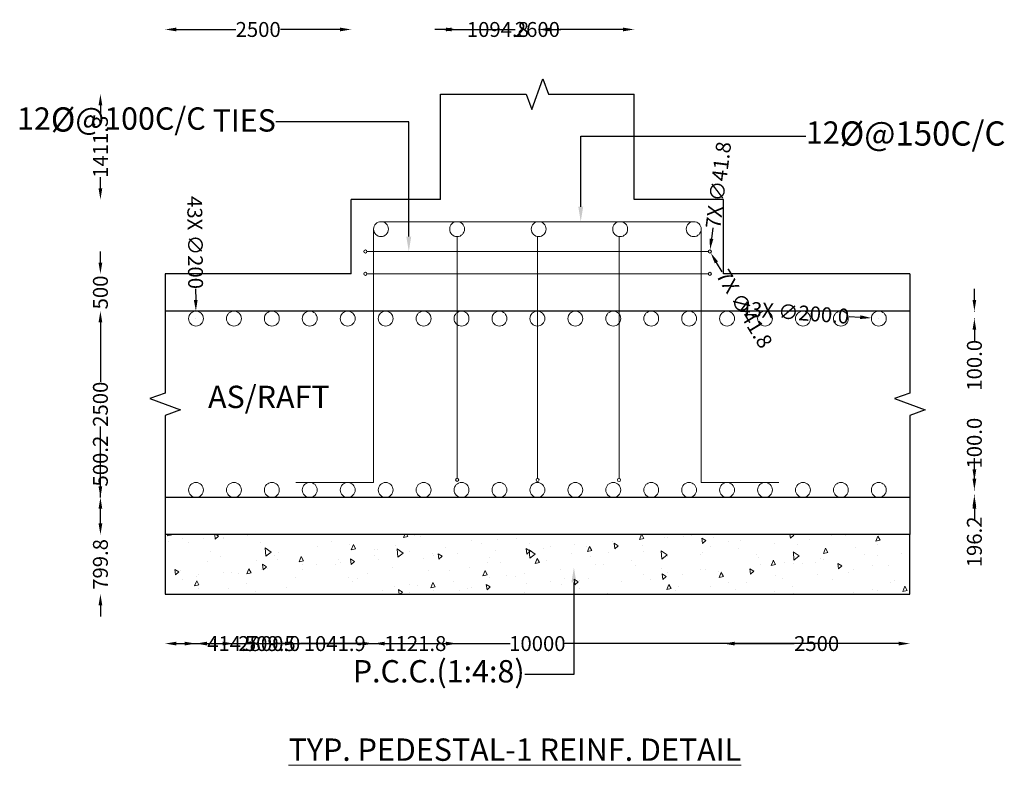
# Model space of a CAD drawing. Units: millimetres. Extents: x -30630 to 20484, y 3580 to 30715.
# Tile 3 of 4: x 7261 to 20484, y 4006 to 14014. Entities that reach past the tile are written whole.
import ezdxf
from ezdxf import colors
from ezdxf.entities.mleader import LeaderData, LeaderLine
from ezdxf.math import Vec2, Vec3

# ---------------------------------------------------------------- set-up
doc = ezdxf.new("R2010")
doc.units = ezdxf.units.MM
doc.header["$MEASUREMENT"] = 0
for name, color, linetype, lineweight in [('S-ANNO-DIMS', 2, 'Continuous', 18), ('S-ANNO-TEXT', 7, 'Continuous', 18), ('S-CONC', 7, 'Continuous', 25), ('S-FNDN-PATT', 8, 'Continuous', 13), ('S-REIN', 1, 'Continuous', 18)]:
    doc.layers.add(name, color=color, linetype=linetype, lineweight=lineweight)
doc.styles.get("Standard").update_dxf_attribs({"font": 'arial.ttf'})
doc.dimstyles.get("Standard").update_dxf_attribs({"dimtxt": 200, "dimasz": 150, "dimexe": 0.18, "dimexo": 0.0625, "dimgap": 0.09, "dimtad": 0, "dimdec": 0, "dimzin": 0, "dimdsep": 46, "dimtxsty": 'Standard', "dimcen": 0.09, "dimadec": 0, "dimazin": 0, "dimtfac": 1, "dimtdec": 0, "dimtofl": 0, "dimtmove": 0, "dimatfit": 3, "dimfxl": 1, "dimfxlon": 1, "dimtolj": 1, "dimtzin": 0, "dimarcsym": 0})

# ---------------------------------------------------------------- blocks, each defined once
blk = doc.blocks.new('*D49')
at = {"layer": 'Defpoints', "color": 0, "transparency": 16777216}
for p in [(9213, 6302), (19213, 6302), (19213, 5640)]:
    blk.add_point(p, dxfattribs=at)
at = {"layer": 'S-ANNO-DIMS', "color": 0, "lineweight": -2, "transparency": 16777216}
for p, q in [((9213, 5641), (9213, 5640)), ((9363, 5640), (13847, 5640)), ((19063, 5640), (14580, 5640)), ((19213, 5641), (19213, 5640))]:
    blk.add_line(p, q, dxfattribs=at)
at = {"layer": 'S-ANNO-DIMS', "color": 0, "transparency": 16777216}
for points in [[(9363, 5665), (9363, 5615), (9213, 5640)], [(19063, 5665), (19063, 5615), (19213, 5640)]]:
    blk.add_solid(points, dxfattribs=at)
at = {"layer": 'S-ANNO-DIMS', "color": 0, "transparency": 16777216, "insert": (14213, 5640), "char_height": 200, "attachment_point": 5}
blk.add_mtext('\\A1;10000', dxfattribs=at)
blk = doc.blocks.new('*D50')
at = {"layer": 'Defpoints', "color": 0, "transparency": 16777216}
for p in [(8344.880092, 7102.317027), (9213.440898, 7102.317027), (9213.440898, 6302.497027)]:
    blk.add_point(p, dxfattribs=at)
at = {"layer": 'S-ANNO-DIMS', "color": 0, "lineweight": -2, "transparency": 16777216}
for p, q in [((8344.880092, 7252.317027), (8344.880092, 7402.317027)), ((8345.880092, 7102.317027), (8344.700092, 7102.317027)), ((8345.880092, 6302.497027), (8344.700092, 6302.497027)), ((8344.880092, 6152.497027), (8344.880092, 6002.497027))]:
    blk.add_line(p, q, dxfattribs=at)
at = {"layer": 'S-ANNO-DIMS', "color": 0, "transparency": 16777216}
for points in [[(8319.880092, 7252.317027), (8369.880092, 7252.317027), (8344.880092, 7102.317027)], [(8319.880092, 6152.497027), (8369.880092, 6152.497027), (8344.880092, 6302.497027)]]:
    blk.add_solid(points, dxfattribs=at)
at = {"layer": 'S-ANNO-DIMS', "color": 0, "transparency": 16777216, "insert": (8344.880092, 6702.407027), "char_height": 200, "attachment_point": 5, "rotation": 90}
blk.add_mtext('\\A1;799.8', dxfattribs=at)
blk = doc.blocks.new('*D51')
at = {"layer": 'Defpoints', "color": 0, "transparency": 16777216}
for p in [(8345, 7602), (9213, 7602), (9213, 7102)]:
    blk.add_point(p, dxfattribs=at)
at = {"layer": 'S-ANNO-DIMS', "color": 0, "lineweight": -2, "transparency": 16777216}
for p, q in [((8345, 7602), (8345, 7752)), ((8346, 7602), (8345, 7602)), ((8345, 7252), (8345, 7452)), ((8346, 7102), (8345, 7102))]:
    blk.add_line(p, q, dxfattribs=at)
at = {"layer": 'S-ANNO-DIMS', "color": 0, "transparency": 16777216}
for points in [[(8320, 7452), (8370, 7452), (8345, 7602)], [(8320, 7252), (8370, 7252), (8345, 7102)]]:
    blk.add_solid(points, dxfattribs=at)
at = {"layer": 'S-ANNO-DIMS', "color": 0, "transparency": 16777216, "insert": (8345, 8089), "char_height": 200, "attachment_point": 5, "rotation": 90}
blk.add_mtext('\\A1;500.2', dxfattribs=at)
blk = doc.blocks.new('*D52')
at = {"layer": 'Defpoints', "color": 0, "transparency": 16777216}
for p in [(8344.880092, 10102.497027), (9213.440898, 10102.497027), (9213.440898, 7602.497027)]:
    blk.add_point(p, dxfattribs=at)
at = {"layer": 'S-ANNO-DIMS', "color": 0, "lineweight": -2, "transparency": 16777216}
for p, q in [((8345.880092, 10102.497027), (8344.700092, 10102.497027)), ((8344.880092, 9952.497027), (8344.880092, 9152.587027)), ((8344.880092, 7752.497027), (8344.880092, 8552.407027)), ((8345.880092, 7602.497027), (8344.700092, 7602.497027))]:
    blk.add_line(p, q, dxfattribs=at)
at = {"layer": 'S-ANNO-DIMS', "color": 0, "transparency": 16777216}
for points in [[(8319.880092, 9952.497027), (8369.880092, 9952.497027), (8344.880092, 10102.497027)], [(8319.880092, 7752.497027), (8369.880092, 7752.497027), (8344.880092, 7602.497027)]]:
    blk.add_solid(points, dxfattribs=at)
at = {"layer": 'S-ANNO-DIMS', "color": 0, "transparency": 16777216, "insert": (8344.880092, 8852.497027), "char_height": 200, "attachment_point": 5, "rotation": 90}
blk.add_mtext('\\A1;2500', dxfattribs=at)
blk = doc.blocks.new('*D53')
at = {"layer": 'Defpoints', "color": 0, "transparency": 16777216}
for p in [(8344.880092, 10602.497027), (9213.440898, 10602.497027), (9213.440898, 10102.497027)]:
    blk.add_point(p, dxfattribs=at)
at = {"layer": 'S-ANNO-DIMS', "color": 0, "lineweight": -2, "transparency": 16777216}
for p, q in [((8344.880092, 10752.497027), (8344.880092, 10902.497027)), ((8345.880092, 10602.497027), (8344.700092, 10602.497027)), ((8345.880092, 10102.497027), (8344.700092, 10102.497027)), ((8344.880092, 9952.497027), (8344.880092, 9802.497027))]:
    blk.add_line(p, q, dxfattribs=at)
at = {"layer": 'S-ANNO-DIMS', "color": 0, "transparency": 16777216}
for points in [[(8319.880092, 10752.497027), (8369.880092, 10752.497027), (8344.880092, 10602.497027)], [(8319.880092, 9952.497027), (8369.880092, 9952.497027), (8344.880092, 10102.497027)]]:
    blk.add_solid(points, dxfattribs=at)
at = {"layer": 'S-ANNO-DIMS', "color": 0, "transparency": 16777216, "insert": (8344.880092, 10352.497027), "char_height": 200, "attachment_point": 5, "rotation": 90}
blk.add_mtext('\\A1;500', dxfattribs=at)
blk = doc.blocks.new('*D54')
at = {"layer": 'Defpoints', "color": 0, "transparency": 16777216}
for p in [(8345, 13014), (12913, 13014), (12913, 11602)]:
    blk.add_point(p, dxfattribs=at)
at = {"layer": 'S-ANNO-DIMS', "color": 0, "lineweight": -2, "transparency": 16777216}
for p, q in [((8346, 13014), (8345, 13014)), ((8345, 12864), (8345, 12714)), ((8345, 11752), (8345, 11902)), ((8346, 11602), (8345, 11602))]:
    blk.add_line(p, q, dxfattribs=at)
at = {"layer": 'S-ANNO-DIMS', "color": 0, "transparency": 16777216}
for points in [[(8320, 12864), (8370, 12864), (8345, 13014)], [(8320, 11752), (8370, 11752), (8345, 11602)]]:
    blk.add_solid(points, dxfattribs=at)
at = {"layer": 'S-ANNO-DIMS', "color": 0, "transparency": 16777216, "insert": (8345, 12308), "char_height": 200, "attachment_point": 5, "rotation": 90}
blk.add_mtext('\\A1;1411.3', dxfattribs=at)
blk = doc.blocks.new('*D55')
at = {"layer": 'Defpoints', "color": 0, "transparency": 16777216}
for p in [(11713.440898, 13882.39252), (9213.440898, 10602.497027), (11713.440898, 10602.497027)]:
    blk.add_point(p, dxfattribs=at)
at = {"layer": 'S-ANNO-DIMS', "color": 0, "lineweight": -2, "transparency": 16777216}
for p, q in [((9213.440898, 13881.39252), (9213.440898, 13882.57252)), ((9363.440898, 13882.39252), (10163.350898, 13882.39252)), ((11563.440898, 13882.39252), (10763.530898, 13882.39252)), ((11713.440898, 13881.39252), (11713.440898, 13882.57252))]:
    blk.add_line(p, q, dxfattribs=at)
at = {"layer": 'S-ANNO-DIMS', "color": 0, "transparency": 16777216}
for points in [[(9363.440898, 13907.39252), (9363.440898, 13857.39252), (9213.440898, 13882.39252)], [(11563.440898, 13907.39252), (11563.440898, 13857.39252), (11713.440898, 13882.39252)]]:
    blk.add_solid(points, dxfattribs=at)
at = {"layer": 'S-ANNO-DIMS', "color": 0, "transparency": 16777216, "insert": (10463.440898, 13882.39252), "char_height": 200, "attachment_point": 5}
blk.add_mtext('\\A1;2500', dxfattribs=at)
blk = doc.blocks.new('*D56')
at = {"layer": 'Defpoints', "color": 0, "transparency": 16777216}
for p in [(15513.620898, 13882.39252), (12913.440898, 13013.831714), (15513.620898, 13013.831714)]:
    blk.add_point(p, dxfattribs=at)
at = {"layer": 'S-ANNO-DIMS', "color": 0, "lineweight": -2, "transparency": 16777216}
for p, q in [((12913.440898, 13881.39252), (12913.440898, 13882.57252)), ((13063.440898, 13882.39252), (13913.440898, 13882.39252)), ((15363.620898, 13882.39252), (14513.620898, 13882.39252)), ((15513.620898, 13881.39252), (15513.620898, 13882.57252))]:
    blk.add_line(p, q, dxfattribs=at)
at = {"layer": 'S-ANNO-DIMS', "color": 0, "transparency": 16777216}
for points in [[(13063.440898, 13907.39252), (13063.440898, 13857.39252), (12913.440898, 13882.39252)], [(15363.620898, 13907.39252), (15363.620898, 13857.39252), (15513.620898, 13882.39252)]]:
    blk.add_solid(points, dxfattribs=at)
at = {"layer": 'S-ANNO-DIMS', "color": 0, "transparency": 16777216, "insert": (14213.530898, 13882.39252), "char_height": 200, "attachment_point": 5}
blk.add_mtext('\\A1;2600', dxfattribs=at)
blk = doc.blocks.new('*D57')
at = {"layer": 'Defpoints', "color": 0, "transparency": 16777216}
for p in [(16713.440898, 10602.497027), (19213.440898, 10602.497027), (19213.440898, 5639.997027)]:
    blk.add_point(p, dxfattribs=at)
at = {"layer": 'S-ANNO-DIMS', "color": 0, "lineweight": -2, "transparency": 16777216}
for p, q in [((16713.440898, 5640.997027), (16713.440898, 5639.817027)), ((16863.440898, 5639.997027), (17663.350898, 5639.997027)), ((19063.440898, 5639.997027), (18263.530898, 5639.997027)), ((19213.440898, 5640.997027), (19213.440898, 5639.817027))]:
    blk.add_line(p, q, dxfattribs=at)
at = {"layer": 'S-ANNO-DIMS', "color": 0, "transparency": 16777216}
for points in [[(16863.440898, 5664.997027), (16863.440898, 5614.997027), (16713.440898, 5639.997027)], [(19063.440898, 5664.997027), (19063.440898, 5614.997027), (19213.440898, 5639.997027)]]:
    blk.add_solid(points, dxfattribs=at)
at = {"layer": 'S-ANNO-DIMS', "color": 0, "transparency": 16777216, "insert": (17963.440898, 5639.997027), "char_height": 200, "attachment_point": 5}
blk.add_mtext('\\A1;2500', dxfattribs=at)
blk = doc.blocks.new('*D58')
at = {"layer": 'Defpoints', "color": 0, "transparency": 16777216}
for p in [(9628, 7702), (10138, 7702), (10138, 5640)]:
    blk.add_point(p, dxfattribs=at)
at = {"layer": 'S-ANNO-DIMS', "color": 0, "lineweight": -2, "transparency": 16777216}
for p, q in [((9628, 5641), (9628, 5640)), ((9778, 5640), (9988, 5640)), ((10138, 5641), (10138, 5640)), ((10138, 5640), (10288, 5640))]:
    blk.add_line(p, q, dxfattribs=at)
at = {"layer": 'S-ANNO-DIMS', "color": 0, "transparency": 16777216}
for points in [[(9778, 5665), (9778, 5615), (9628, 5640)], [(9988, 5665), (9988, 5615), (10138, 5640)]]:
    blk.add_solid(points, dxfattribs=at)
at = {"layer": 'S-ANNO-DIMS', "color": 0, "transparency": 16777216, "insert": (10626, 5640), "char_height": 200, "attachment_point": 5}
blk.add_mtext('\\A1;509.5', dxfattribs=at)
blk = doc.blocks.new('*D59')
at = {"layer": 'Defpoints', "color": 0, "transparency": 16777216}
for p in [(14230.091081, 13882.39252), (13135.266383, 11202.497027), (14230.091081, 11202.497027)]:
    blk.add_point(p, dxfattribs=at)
at = {"layer": 'S-ANNO-DIMS', "color": 0, "lineweight": -2, "transparency": 16777216}
for p, q in [((12985.266383, 13882.39252), (12835.266383, 13882.39252)), ((13135.266383, 13881.39252), (13135.266383, 13882.57252)), ((14230.091081, 13881.39252), (14230.091081, 13882.57252)), ((14380.091081, 13882.39252), (14530.091081, 13882.39252))]:
    blk.add_line(p, q, dxfattribs=at)
at = {"layer": 'S-ANNO-DIMS', "color": 0, "transparency": 16777216}
for points in [[(12985.266383, 13907.39252), (12985.266383, 13857.39252), (13135.266383, 13882.39252)], [(14380.091081, 13907.39252), (14380.091081, 13857.39252), (14230.091081, 13882.39252)]]:
    blk.add_solid(points, dxfattribs=at)
at = {"layer": 'S-ANNO-DIMS', "color": 0, "transparency": 16777216, "insert": (13682.678732, 13882.39252), "char_height": 200, "attachment_point": 5}
blk.add_mtext('\\A1;1094.8', dxfattribs=at)
blk = doc.blocks.new('*D62')
at = {"layer": 'Defpoints', "color": 0, "transparency": 16777216}
for p in [(9627, 10102), (9629, 9903)]:
    blk.add_point(p, dxfattribs=at)
at = {"layer": 'S-ANNO-DIMS', "color": 0, "lineweight": -2, "transparency": 16777216}
for p, q in [((9624, 10402), (9625, 10252)), ((9628, 10002), (9628, 10003)), ((9628, 10002), (9628, 10002))]:
    blk.add_line(p, q, dxfattribs=at)
at = {"layer": 'S-ANNO-DIMS', "color": 0, "transparency": 16777216}
blk.add_solid([(9650, 10253), (9600, 10252), (9627, 10102)], dxfattribs=at)
at = {"layer": 'S-ANNO-DIMS', "color": 0, "transparency": 16777216, "insert": (9617, 11023), "char_height": 200, "attachment_point": 5, "rotation": 270.6269}
blk.add_mtext('\\A1;43X ∅200', dxfattribs=at)
blk = doc.blocks.new('*D63')
at = {"layer": 'Defpoints', "color": 0, "transparency": 16777216}
for p in [(16526, 10882), (16532, 10923)]:
    blk.add_point(p, dxfattribs=at)
at = {"layer": 'S-ANNO-DIMS', "color": 0, "lineweight": -2, "transparency": 16777216}
for p, q in [((16570, 11221), (16551, 11072)), ((16529, 10902), (16529, 10903)), ((16529, 10902), (16529, 10902))]:
    blk.add_line(p, q, dxfattribs=at)
at = {"layer": 'S-ANNO-DIMS', "color": 0, "transparency": 16777216}
blk.add_solid([(16526, 11075), (16576, 11069), (16532, 10923)], dxfattribs=at)
at = {"layer": 'S-ANNO-DIMS', "color": 0, "transparency": 16777216, "insert": (16644, 11794), "char_height": 200, "attachment_point": 5, "rotation": 82.6437}
blk.add_mtext('\\A1;7X ∅41.8', dxfattribs=at)
blk = doc.blocks.new('*D73')
at = {"layer": 'Defpoints', "color": 0, "transparency": 16777216}
for p in [(9628.132508, 7702.497027), (9213.440898, 7602.497027), (9628.132508, 5639.997027)]:
    blk.add_point(p, dxfattribs=at)
at = {"layer": 'S-ANNO-DIMS', "color": 0, "lineweight": -2, "transparency": 16777216}
for p, q in [((9213.440898, 5640.997027), (9213.440898, 5639.817027)), ((9363.440898, 5639.997027), (9478.132508, 5639.997027)), ((9628.132508, 5640.997027), (9628.132508, 5639.817027)), ((9628.132508, 5639.997027), (9778.132508, 5639.997027))]:
    blk.add_line(p, q, dxfattribs=at)
at = {"layer": 'S-ANNO-DIMS', "color": 0, "transparency": 16777216}
for points in [[(9363.440898, 5664.997027), (9363.440898, 5614.997027), (9213.440898, 5639.997027)], [(9478.132508, 5664.997027), (9478.132508, 5614.997027), (9628.132508, 5639.997027)]]:
    blk.add_solid(points, dxfattribs=at)
at = {"layer": 'S-ANNO-DIMS', "color": 0, "transparency": 16777216, "insert": (10119.695905, 5639.997027), "char_height": 200, "attachment_point": 5}
blk.add_mtext('\\A1;414.7', dxfattribs=at)
blk = doc.blocks.new('*D74')
at = {"layer": 'Defpoints', "color": 0, "transparency": 16777216}
for p in [(19213, 10102), (18798, 10002), (20082, 10002)]:
    blk.add_point(p, dxfattribs=at)
at = {"layer": 'S-ANNO-DIMS', "color": 0, "lineweight": -2, "transparency": 16777216}
for p, q in [((20082, 10252), (20082, 10402)), ((20081, 10102), (20082, 10102)), ((20081, 10002), (20082, 10002)), ((20082, 9852), (20082, 9702))]:
    blk.add_line(p, q, dxfattribs=at)
at = {"layer": 'S-ANNO-DIMS', "color": 0, "transparency": 16777216}
for points in [[(20057, 10252), (20107, 10252), (20082, 10102)], [(20057, 9852), (20107, 9852), (20082, 10002)]]:
    blk.add_solid(points, dxfattribs=at)
at = {"layer": 'S-ANNO-DIMS', "color": 0, "transparency": 16777216, "insert": (20082, 9375), "char_height": 200, "attachment_point": 5, "rotation": 90}
blk.add_mtext('\\A1;100.0', dxfattribs=at)
blk = doc.blocks.new('*D75')
at = {"layer": 'Defpoints', "color": 0, "transparency": 16777216}
for p in [(18798, 7702), (20082, 7702), (19213, 7602)]:
    blk.add_point(p, dxfattribs=at)
at = {"layer": 'S-ANNO-DIMS', "color": 0, "lineweight": -2, "transparency": 16777216}
for p, q in [((20082, 7852), (20082, 8002)), ((20081, 7702), (20082, 7702)), ((20081, 7602), (20082, 7602)), ((20082, 7452), (20082, 7302))]:
    blk.add_line(p, q, dxfattribs=at)
at = {"layer": 'S-ANNO-DIMS', "color": 0, "transparency": 16777216}
for points in [[(20057, 7852), (20107, 7852), (20082, 7702)], [(20057, 7452), (20107, 7452), (20082, 7602)]]:
    blk.add_solid(points, dxfattribs=at)
at = {"layer": 'S-ANNO-DIMS', "color": 0, "transparency": 16777216, "insert": (20082, 8330), "char_height": 200, "attachment_point": 5, "rotation": 90}
blk.add_mtext('\\A1;100.0', dxfattribs=at)
blk = doc.blocks.new('*D76')
at = {"layer": 'Defpoints', "color": 0, "transparency": 16777216}
for p in [(12013, 7802), (9213, 7602), (12013, 5640)]:
    blk.add_point(p, dxfattribs=at)
at = {"layer": 'S-ANNO-DIMS', "color": 0, "lineweight": -2, "transparency": 16777216}
for p, q in [((9213, 5641), (9213, 5640)), ((9363, 5640), (10197, 5640)), ((11863, 5640), (11030, 5640)), ((12013, 5641), (12013, 5640))]:
    blk.add_line(p, q, dxfattribs=at)
at = {"layer": 'S-ANNO-DIMS', "color": 0, "transparency": 16777216}
for points in [[(9363, 5665), (9363, 5615), (9213, 5640)], [(11863, 5665), (11863, 5615), (12013, 5640)]]:
    blk.add_solid(points, dxfattribs=at)
at = {"layer": 'S-ANNO-DIMS', "color": 0, "transparency": 16777216, "insert": (10613, 5640), "char_height": 200, "attachment_point": 5}
blk.add_mtext('\\A1;2800.0', dxfattribs=at)
blk = doc.blocks.new('*D77')
at = {"layer": 'Defpoints', "color": 0, "transparency": 16777216}
for p in [(10972, 7802), (12013, 7802), (12013, 5640)]:
    blk.add_point(p, dxfattribs=at)
at = {"layer": 'S-ANNO-DIMS', "color": 0, "lineweight": -2, "transparency": 16777216}
for p, q in [((10822, 5640), (10672, 5640)), ((10972, 5641), (10972, 5640)), ((12013, 5641), (12013, 5640)), ((12163, 5640), (12313, 5640))]:
    blk.add_line(p, q, dxfattribs=at)
at = {"layer": 'S-ANNO-DIMS', "color": 0, "transparency": 16777216}
for points in [[(10822, 5665), (10822, 5615), (10972, 5640)], [(12163, 5665), (12163, 5615), (12013, 5640)]]:
    blk.add_solid(points, dxfattribs=at)
at = {"layer": 'S-ANNO-DIMS', "color": 0, "transparency": 16777216, "insert": (11492, 5640), "char_height": 200, "attachment_point": 5}
blk.add_mtext('\\A1;1041.9', dxfattribs=at)
blk = doc.blocks.new('*D78')
at = {"layer": 'Defpoints', "color": 0, "transparency": 16777216}
for p in [(12013, 7802), (13135, 7837), (13135, 5640)]:
    blk.add_point(p, dxfattribs=at)
at = {"layer": 'S-ANNO-DIMS', "color": 0, "lineweight": -2, "transparency": 16777216}
for p, q in [((12013, 5641), (12013, 5640)), ((12163, 5640), (12168, 5640)), ((12985, 5640), (12980, 5640)), ((13135, 5641), (13135, 5640))]:
    blk.add_line(p, q, dxfattribs=at)
at = {"layer": 'S-ANNO-DIMS', "color": 0, "transparency": 16777216}
for points in [[(12163, 5665), (12163, 5615), (12013, 5640)], [(12985, 5665), (12985, 5615), (13135, 5640)]]:
    blk.add_solid(points, dxfattribs=at)
at = {"layer": 'S-ANNO-DIMS', "color": 0, "transparency": 16777216, "insert": (12574, 5640), "char_height": 200, "attachment_point": 5}
blk.add_mtext('\\A1;1121.8', dxfattribs=at)
blk = doc.blocks.new('*D79')
at = {"layer": 'Defpoints', "color": 0, "transparency": 16777216}
for p in [(15330, 7828), (15303, 7632), (20082, 7632)]:
    blk.add_point(p, dxfattribs=at)
at = {"layer": 'S-ANNO-DIMS', "color": 0, "lineweight": -2, "transparency": 16777216}
for p, q in [((20082, 7978), (20082, 8128)), ((20081, 7828), (20082, 7828)), ((20081, 7632), (20082, 7632)), ((20082, 7482), (20082, 7332))]:
    blk.add_line(p, q, dxfattribs=at)
at = {"layer": 'S-ANNO-DIMS', "color": 0, "transparency": 16777216}
for points in [[(20057, 7978), (20107, 7978), (20082, 7828)], [(20057, 7482), (20107, 7482), (20082, 7632)]]:
    blk.add_solid(points, dxfattribs=at)
at = {"layer": 'S-ANNO-DIMS', "color": 0, "transparency": 16777216, "insert": (20082, 7005), "char_height": 200, "attachment_point": 5, "rotation": 90}
blk.add_mtext('\\A1;196.2', dxfattribs=at)
blk = doc.blocks.new('*D82')
at = {"layer": 'Defpoints', "color": 0, "transparency": 16777216}
for p in [(18699, 10010), (18898, 9995)]:
    blk.add_point(p, dxfattribs=at)
at = {"layer": 'S-ANNO-DIMS', "color": 0, "lineweight": -2, "transparency": 16777216}
for p, q in [((18399, 10031), (18549, 10021)), ((18798, 10002), (18798, 10003)), ((18798, 10002), (18799, 10002))]:
    blk.add_line(p, q, dxfattribs=at)
at = {"layer": 'S-ANNO-DIMS', "color": 0, "transparency": 16777216}
blk.add_solid([(18551, 10046), (18547, 9996), (18699, 10010)], dxfattribs=at)
at = {"layer": 'S-ANNO-DIMS', "color": 0, "transparency": 16777216, "insert": (17664, 10085), "char_height": 200, "attachment_point": 5, "rotation": 355.842}
blk.add_mtext('\\A1;43X ∅200.0', dxfattribs=at)
blk = doc.blocks.new('*D83')
at = {"layer": 'Defpoints', "color": 0, "transparency": 16777216}
for p in [(16518, 10920), (16540, 10885)]:
    blk.add_point(p, dxfattribs=at)
at = {"layer": 'S-ANNO-DIMS', "color": 0, "lineweight": -2, "transparency": 16777216}
for p, q in [((16529, 10902), (16529, 10903)), ((16529, 10902), (16529, 10902)), ((16695, 10628), (16618, 10756))]:
    blk.add_line(p, q, dxfattribs=at)
at = {"layer": 'S-ANNO-DIMS', "color": 0, "transparency": 16777216}
blk.add_solid([(16639, 10769), (16596, 10743), (16540, 10885)], dxfattribs=at)
at = {"layer": 'S-ANNO-DIMS', "color": 0, "transparency": 16777216, "insert": (16994, 10134), "char_height": 200, "attachment_point": 5, "rotation": 301.1587}
blk.add_mtext('\\A1;7X ∅41.8', dxfattribs=at)

msp = doc.modelspace()

# ---------------------------------------------------------------- hatches: boundary and pattern name
at = {"layer": 'S-FNDN-PATT'}
h = msp.add_hatch(dxfattribs=at)
h.set_pattern_fill('AR-CONC', color=256, scale=100, angle=47)
h.set_pattern_definition([(97, (-22147.15, -7912.8), (535.064, 481.774), [75, -825]), (42, (-22147.15, -7912.8), (-644.747, 411.518), [60, -660]), (147.4514, (-22102.56, -7872.64), (-109.682, 893.292), [63.74, -701.142]), (93.1842, (-22293.4, -7776.4), (848.91, 667.647), [112.5, -1237.5]), (143.6356, (-22222.7, -7720.8), (-74.987, 1347.916), [95.61, -1051.714]), (38.1842, (-22293.4, -7776.4), (-74.987, 1347.916), [90, -990]), (68, (-22188.65, -7737.35), (701.5464, 161.965), [75, -825]), (13, (-22188.65, -7737.35), (-364.4, 672.501), [60, -660]), (118.4514, (-22130.2, -7723.86), (337.146, 834.465), [63.74, -701.142]), (84.5, (-22147.15, -7912.8), (-235.1702, 235.9262), [0, -652, 0, -670, 0, -662.5]), (54.5, (-22147.15, -7912.8), (-109.0415, 461.385), [0, -382, 0, -637, 0, -252.5]), (14.5, (-22299.23, -8075.88), (380.5616, 375.0306), [0, -250, 0, -780, 0, -1035]), (4.5, (-22367.43, -8149), (324.52, 494.787), [0, -325, 0, -518, 0, -735])])
h.paths.add_polyline_path([(9213.4409, 7102.497), (9213.4409, 7102.317), (9213.4409, 6302.497), (19213.4409, 6302.497), (19213.4409, 7102.497)])

# ---------------------------------------------------------------- linework, layer by layer
at = {"layer": 'S-CONC'}
for p, q in [((12913.4409, 11602.497), (12913.4409, 13013.8317)), ((15513.4409, 11602.497), (15513.4409, 13013.8317)), ((11713.4409, 10602.497), (11713.4409, 11602.497)), ((12913.4409, 11602.497), (11713.4409, 11602.497)), ((16713.4409, 11602.497), (15513.4409, 11602.497)), ((16713.4409, 10602.497), (16713.4409, 11602.497)), ((11713.4409, 10602.497), (9213.4409, 10602.497)), ((19213.4409, 10602.497), (16713.4409, 10602.497)), ((19213.4409, 10102.497), (9213.4409, 10102.497)), ((19213.4409, 7602.497), (9213.4409, 7602.497)), ((19213.4409, 7102.497), (9213.4409, 7102.497)), ((9213.4409, 7102.497), (9213.4409, 6302.497)), ((19213.4409, 6302.497), (19213.4409, 7102.497)), ((9213.4409, 6302.497), (19213.4409, 6302.497))]:
    msp.add_line(p, q, dxfattribs=at)
for points in [[(12913.2609, 13013.8317), (14063.4409, 13013.8317), (14138.4409, 12807.7709), (14288.4409, 13219.8925), (14363.4409, 13013.8317), (15513.6209, 13013.8317)], [(9213.4409, 10602.677), (9213.4409, 9002.497), (9007.3801, 8927.497), (9419.5017, 8777.497), (9213.4409, 8702.497), (9213.4409, 7102.317)], [(19213.4409, 10602.677), (19213.4409, 9002.497), (19007.3801, 8927.497), (19419.5017, 8777.497), (19213.4409, 8702.497), (19213.4409, 7102.317)]]:
    msp.add_lwpolyline(points, dxfattribs=at)
at = {"layer": 'S-REIN'}
for p, q in [((16313.4409, 11302.497), (12113.4409, 11302.497)), ((12013.4409, 10602.497), (12013.4409, 11202.497)), ((16413.4409, 10602.497), (16413.4409, 11202.497)), ((13135.2664, 11102.497), (13135.2664, 7858.0868)), ((14215.5679, 11101.4368), (14215.5679, 7857.0266)), ((15310.3439, 11101.4368), (15310.3439, 7857.0266)), ((11924.3043, 10902.497), (16508.1966, 10902.497)), ((11924.3043, 10602.497), (16508.1966, 10602.497)), ((12013.4409, 10602.497), (12013.4409, 7802.497)), ((16413.4409, 10602.497), (16413.4409, 7802.497)), ((12013.4409, 7802.497), (10971.5117, 7802.497)), ((16413.4409, 7802.497), (17455.3701, 7802.497))]:
    msp.add_line(p, q, dxfattribs=at)
for centre, radius in [((12113.4409, 11202.497), 100), ((13135.2664, 11202.497), 100), ((14230.0911, 11202.497), 100), ((15324.9158, 11202.497), 100), ((16313.4409, 11202.497), 100), ((11903.406, 10902.497), 20.8983), ((16529.0948, 10902.497), 20.8983), ((11903.406, 10602.497), 20.8983), ((16529.0948, 10602.497), 20.8983), ((9628.1325, 10002.497), 100), ((10137.5941, 10002.497), 100), ((10647.0557, 10002.497), 100), ((11156.5172, 10002.497), 100), ((11665.9788, 10002.497), 100), ((12175.4404, 10002.497), 100), ((12684.902, 10002.497), 100), ((13194.3635, 10002.497), 100), ((13703.8251, 10002.497), 100), ((14213.2867, 10002.497), 100), ((14722.7483, 10002.497), 100), ((15232.2099, 10002.497), 100), ((15741.6714, 10002.497), 100), ((16251.133, 10002.497), 100), ((16760.5946, 10002.497), 100), ((17270.0562, 10002.497), 100), ((17779.5177, 10002.497), 100), ((18288.9793, 10002.497), 100), ((18798.4409, 10002.497), 100), ((9628.1325, 7702.497), 100), ((10137.5941, 7702.497), 100), ((10647.0557, 7702.497), 100), ((11156.5172, 7702.497), 100), ((11665.9788, 7702.497), 100), ((12175.4404, 7702.497), 100), ((12684.902, 7702.497), 100), ((13194.3635, 7702.497), 100), ((13135.2664, 7837.1885), 20.8983), ((13703.8251, 7702.497), 100), ((14213.2867, 7702.497), 100), ((14215.5679, 7836.1283), 20.8983), ((14722.7483, 7702.497), 100), ((15232.2099, 7702.497), 100), ((15310.3439, 7836.1283), 20.8983), ((15741.6714, 7702.497), 100), ((16251.133, 7702.497), 100), ((16760.5946, 7702.497), 100), ((17270.0562, 7702.497), 100), ((17779.5177, 7702.497), 100), ((18288.9793, 7702.497), 100), ((18798.4409, 7702.497), 100)]:
    msp.add_circle(centre, radius, dxfattribs=at)

# ---------------------------------------------------------------- texts
at = {"layer": 'S-ANNO-TEXT', "char_height": 300, "attachment_point": 1}
for s, width, insert in [('{\\fArial|b1|i0|c0|p34;AS/RAFT}', 1058.385802, (9790.418, 9101.0935)), ('{\\fArial|b1|i0|c0|p34;\\LTYP. PEDESTAL-1 REINF. DETAIL}', 7568.651815, (10871.9893, 4366.329))]:
    msp.add_mtext_dynamic_manual_height_columns(s, width=width, gutter_width=1, heights=[0], dxfattribs=dict(at, insert=insert))

# ---------------------------------------------------------------- dimensions: what is measured, and where the dimension line sits
at = {"layer": 'S-ANNO-DIMS'}
for base, p1, p2, override, picture, middle in [((11713.4409, 13882.3925), (9213.4409, 10602.497), (11713.4409, 10602.497), {"dimdec": 0, "dimlfac": 1, "dimrnd": 0, "dimzin": 0, "dimdsep": 46, "dimlunit": 2}, '*D55', (10463.4409, 13882.3925)), ((14230.0911, 13882.3925), (13135.2664, 11202.497), (14230.0911, 11202.497), {"dimdec": 1, "dimlfac": 1, "dimrnd": 0, "dimzin": 0, "dimdsep": 46, "dimlunit": 2}, '*D59', (13682.6787, 13882.3925)), ((15513.6209, 13882.3925), (12913.4409, 13013.8317), (15513.6209, 13013.8317), {"dimdec": 0, "dimlfac": 1, "dimrnd": 0, "dimzin": 0, "dimdsep": 46, "dimlunit": 2}, '*D56', (14213.5309, 13882.3925)), ((19213.4409, 5639.997), (16713.4409, 10602.497), (19213.4409, 10602.497), {"dimdec": 0, "dimlfac": 1, "dimrnd": 0, "dimzin": 0, "dimdsep": 46, "dimlunit": 2}, '*D57', (17963.4409, 5639.997)), ((12013.4409, 5639.997), (9213.4409, 7602.497), (12013.4409, 7802.497), {"dimdec": 1, "dimlfac": 1, "dimrnd": 0, "dimzin": 0, "dimdsep": 46, "dimlunit": 2}, '*D76', (10613.4409, 5639.997)), ((12013.4409, 5639.997), (10971.5117, 7802.497), (12013.4409, 7802.497), {"dimdec": 1, "dimlfac": 1, "dimrnd": 0, "dimzin": 0, "dimdsep": 46, "dimlunit": 2}, '*D77', (11492.4763, 5639.997)), ((13135.2664, 5639.997), (12013.4409, 7802.497), (13135.2664, 7837.1885), {"dimdec": 1, "dimlfac": 1, "dimrnd": 0, "dimzin": 0, "dimdsep": 46, "dimlunit": 2}, '*D78', (12574.3536, 5639.997)), ((9628.1325, 5639.997), (9213.4409, 7602.497), (9628.1325, 7702.497), {"dimdec": 1, "dimlfac": 1, "dimrnd": 0, "dimzin": 0, "dimdsep": 46, "dimlunit": 2}, '*D73', (10119.6959, 5639.997)), ((10137.5941, 5639.997), (9628.1325, 7702.497), (10137.5941, 7702.497), {"dimdec": 1, "dimlfac": 1, "dimrnd": 0, "dimzin": 0, "dimdsep": 46, "dimlunit": 2}, '*D58', (10625.8833, 5639.997)), ((19213.4409, 5639.997), (9213.4409, 6302.497), (19213.4409, 6302.497), {"dimdec": 0, "dimlfac": 1, "dimrnd": 0, "dimzin": 0, "dimdsep": 46, "dimlunit": 2}, '*D49', (14213.4409, 5639.997))]:
    dim = msp.add_linear_dim(base=base, p1=p1, p2=p2, dimstyle='Standard', override=override, dxfattribs=at)
    dim.commit()
    dim.dimension.update_dxf_attribs({"geometry": picture, "text_midpoint": middle})
for base, p1, p2, override, picture, middle in [((8344.8801, 13013.8317), (12913.4409, 11602.497), (12913.4409, 13013.8317), {"dimdec": 1, "dimlfac": 1, "dimrnd": 0, "dimzin": 0, "dimdsep": 46, "dimlunit": 2}, '*D54', (8344.8801, 12308.1644)), ((8344.8801, 10602.497), (9213.4409, 10102.497), (9213.4409, 10602.497), {"dimdec": 0, "dimlfac": 1, "dimrnd": 0, "dimzin": 0, "dimdsep": 46, "dimlunit": 2}, '*D53', (8344.8801, 10352.497)), ((20082.0017, 10002.497), (19213.4409, 10102.497), (18798.4409, 10002.497), {"dimdec": 1, "dimlfac": 1, "dimrnd": 0, "dimzin": 0, "dimdsep": 46, "dimlunit": 2}, '*D74', (20082.0017, 9374.7126)), ((8344.8801, 10102.497), (9213.4409, 7602.497), (9213.4409, 10102.497), {"dimdec": 0, "dimlfac": 1, "dimrnd": 0, "dimzin": 0, "dimdsep": 46, "dimlunit": 2}, '*D52', (8344.8801, 8852.497)), ((20082.0017, 7702.497), (19213.4409, 7602.497), (18798.4409, 7702.497), {"dimdec": 1, "dimlfac": 1, "dimrnd": 0, "dimzin": 0, "dimdsep": 46, "dimlunit": 2}, '*D75', (20082.0017, 8330.2814)), ((8344.8801, 7602.497), (9213.4409, 7102.317), (9213.4409, 7602.497), {"dimdec": 1, "dimlfac": 1, "dimrnd": 0, "dimzin": 0, "dimdsep": 46, "dimlunit": 2}, '*D51', (8344.8801, 8089.0127)), ((20082.0017, 7631.7863), (15329.5998, 7827.9938), (15302.9205, 7631.7863), {"dimdec": 1, "dimlfac": 1, "dimrnd": 0, "dimzin": 0, "dimdsep": 46, "dimlunit": 2}, '*D79', (20082.0017, 7004.6841)), ((8344.8801, 7102.317), (9213.4409, 6302.497), (9213.4409, 7102.317), {"dimdec": 1, "dimlfac": 1, "dimrnd": 0, "dimzin": 0, "dimdsep": 46, "dimlunit": 2}, '*D50', (8344.8801, 6702.407))]:
    dim = msp.add_linear_dim(base=base, p1=p1, p2=p2, angle=90, dimstyle='Standard', override=override, dxfattribs=at)
    dim.commit()
    dim.dimension.update_dxf_attribs({"geometry": picture, "text_midpoint": middle})
for p1, p2, text, override, picture, middle in [((16526.4191, 10881.7708), (16531.7706, 10923.2233), '7X <>', {"dimdec": 1, "dimlfac": 1, "dimrnd": 0, "dimzin": 0, "dimdsep": 46, "dimlunit": 2}, '*D63', (16644.1346, 11793.5799)), ((9629.2266, 9902.503), (9627.0384, 10102.491), '43X <>', {"dimdec": 0, "dimlfac": 1, "dimrnd": 0, "dimzin": 0, "dimdsep": 46, "dimlunit": 2}, '*D62', (9616.9642, 11023.1944))]:
    dim = msp.add_diameter_dim_2p(p1=p1, p2=p2, text=text, dimstyle='Standard', override=override, dxfattribs=at)
    dim.commit()
    dim.dimension.update_dxf_attribs({"geometry": picture, "text_midpoint": middle, "dimtype": 163})
for p1, p2, text, picture, middle in [((16518.2819, 10920.3805), (16539.9078, 10884.6136), '7X <>', '*D83', (16993.9768, 10133.6358)), ((18898.1777, 9995.2464), (18698.7041, 10009.7477), '43X <>', '*D82', (17664.1683, 10084.9562))]:
    dim = msp.add_diameter_dim_2p(p1=p1, p2=p2, text=text, dimstyle='Standard', override={"dimdec": 1, "dimlfac": 1, "dimrnd": 0, "dimzin": 0, "dimdsep": 46, "dimlunit": 2}, dxfattribs=at)
    dim.commit()
    dim.dimension.update_dxf_attribs({"geometry": picture, "text_midpoint": middle})

# ---------------------------------------------------------------- leaders
at = {"layer": 'S-ANNO-TEXT'}
ml = msp.add_multileader_mtext('Standard', dxfattribs=at)
ml.set_content('12{\\H1.08333x;Ø}@100C/C TIES', color=256)
ml.set_leader_properties()
ml.build(insert=Vec2(0, 0))
ml.multileader.update_dxf_attribs({"dogleg_length": 0.36, "arrow_head_size": 200})
ctx = ml.context
ctx.base_point, ctx.char_height, ctx.arrow_head_size, ctx.landing_gap_size, ctx.plane_origin = Vec3(7054.8698, 12642.6807), 300, 200, 0.09, Vec3(12486.2719, 10902.497)
ctx.text_align_type = 2
notes = []
notes.append((ctx, [(0, (1, 1, 0), (10701.6059, 12642.6807), (-1, 0), 0.36, [(0, [(12486.2719, 10902.497), (12486.2719, 12642.6807)], 0, [])])]))
ctx.mtext.insert, ctx.mtext.alignment, ctx.mtext.flow_direction = Vec3(10701.1559, 12836.7803), 3, 5
ml = msp.add_multileader_mtext('Standard', dxfattribs=at)
ml.set_content('12{\\H1.08333x;Ø@150C/C}', color=256)
ml.set_leader_properties()
ml.build(insert=Vec2(0, 0))
ml.multileader.update_dxf_attribs({"dogleg_length": 0.36, "arrow_head_size": 200})
ctx = ml.context
ctx.base_point, ctx.char_height, ctx.arrow_head_size, ctx.landing_gap_size, ctx.plane_origin = Vec3(17819.1892, 12450.803), 300, 200, 0.09, Vec3(14795.551, 11302.497)
notes.append((ctx, [(0, (1, 1, 0), (17818.8292, 12450.803), (1, 0), 0.36, [(0, [(14795.551, 11302.497), (14795.551, 12450.803)], 0, [])])]))
ctx.mtext.insert, ctx.mtext.width, ctx.mtext.flow_direction = Vec3(17819.2792, 12648.5774), 2458.179759, 5
ml = msp.add_multileader_mtext('Standard', dxfattribs=at)
ml.set_content('P.C.C.(1:4:8)', color=256)
ml.set_leader_properties()
ml.build(insert=Vec2(0, 0))
ml.multileader.update_dxf_attribs({"dogleg_length": 0.36, "arrow_head_size": 200})
ctx = ml.context
ctx.base_point, ctx.char_height, ctx.arrow_head_size, ctx.landing_gap_size, ctx.plane_origin = Vec3(11644.5165, 5224.076), 300, 200, 0.09, Vec3(14703.5987, 6661.5024)
ctx.text_align_type = 2
notes.append((ctx, [(0, (1, 1, 0), (14043.0101, 5224.076), (-1, 0), 0.36, [(0, [(14703.5987, 6661.5024), (14703.5987, 5224.076)], 0, [])])]))
ctx.mtext.insert, ctx.mtext.alignment, ctx.mtext.flow_direction = Vec3(14042.5601, 5418.1756), 3, 5
for ctx, leaders in notes:
    for number, flags, end, landing, length, lines in leaders:
        leader = LeaderData()
        leader.index, (leader.has_last_leader_line, leader.has_dogleg_vector, leader.attachment_direction) = number, flags
        leader.last_leader_point, leader.dogleg_vector, leader.dogleg_length = Vec3(end), Vec3(landing), length
        for number, points, colour, breaks in lines:
            line = LeaderLine()
            line.index, line.vertices, line.color, line.breaks = number, Vec3.list(points), colors.encode_raw_color(colour), breaks
            leader.lines.append(line)
        ctx.leaders.append(leader)

doc.saveas('drawing.dxf')
